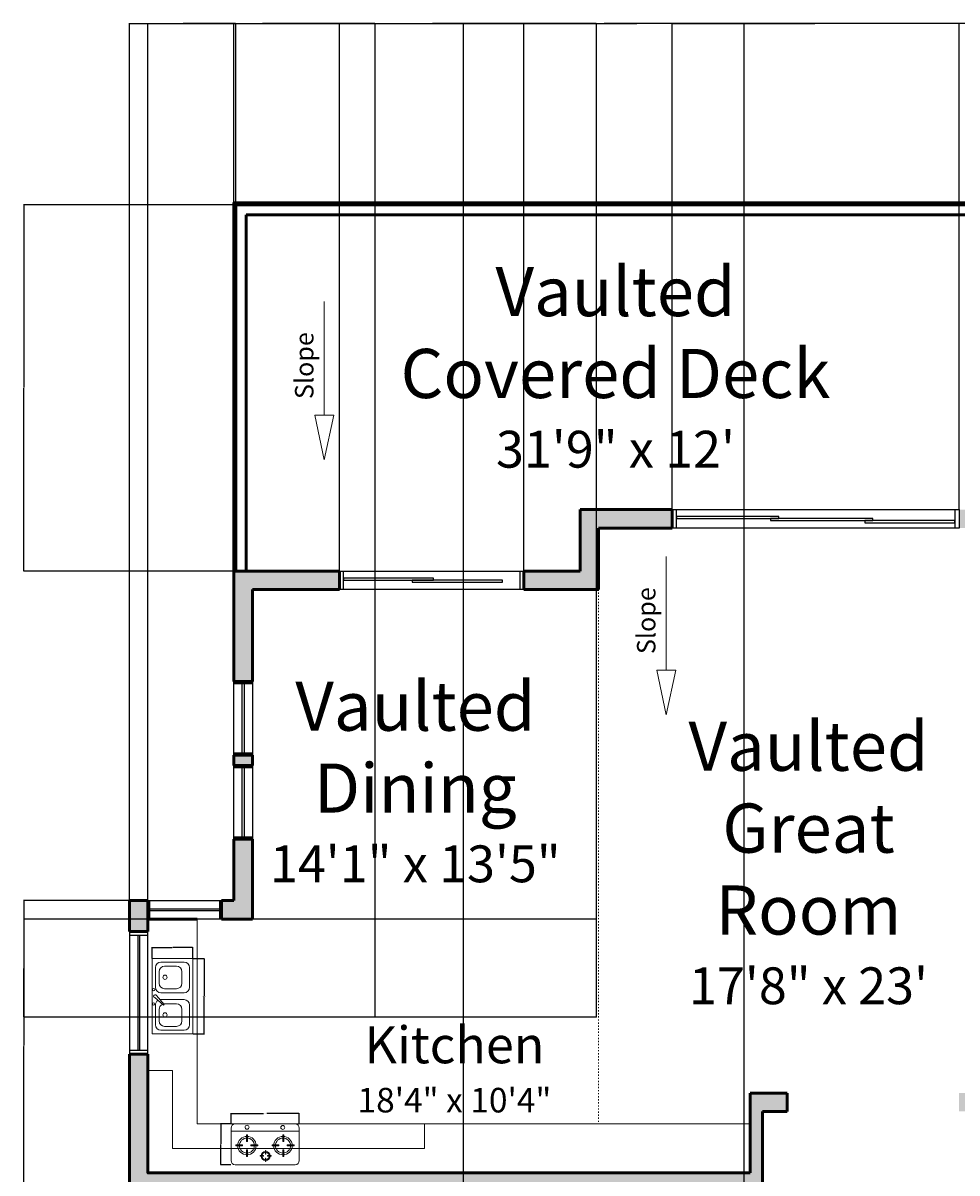
# Model space of a CAD drawing. Units: inches. Extents: x 296 to 2116, y 330 to 1460.
# Tile 3 of 9: x 296 to 752, y 898 to 1460. Entities that reach past the tile are written whole.
import ezdxf

# ---------------------------------------------------------------- set-up
doc = ezdxf.new("R2010")
doc.units = ezdxf.units.IN
doc.linetypes.add('ACAD_ISO03W100', pattern=[30, 12, -18])
for name, color, linetype, lineweight in [('A-ANNO-DIMS', 2, 'Continuous', 18), ('A-ANNO-SYMB', 2, 'Continuous', 18), ('A-ANNO-TEXT', 7, 'Continuous', 18), ('A-AREA-IDEN', 7, 'Continuous', 25), ('A-DOOR', 3, 'Continuous', 25), ('A-FLOR-FIXT', 8, 'Continuous', 18), ('A-FLOR-OVHD', 132, 'ACAD_ISO03W100', 18), ('A-GLAZ', 4, 'Continuous', 25), ('A-WALL', 7, 'Continuous', 50), ('A-WALL-PATT', 8, 'Continuous', 13)]:
    doc.layers.add(name, color=color, linetype=linetype, lineweight=lineweight)
doc.styles.get("Standard").update_dxf_attribs({"font": 'arial.ttf'})
doc.dimstyles.get("Standard").update_dxf_attribs({"dimtxt": 0.18, "dimasz": 0.18, "dimexe": 0.18, "dimexo": 0.0625, "dimgap": 0.09, "dimtad": 0, "dimtih": 1, "dimtoh": 1, "dimdec": 4, "dimzin": 0, "dimdsep": 46, "dimtxsty": 'Standard', "dimcen": 0.09, "dimadec": 0, "dimazin": 0, "dimtfac": 1, "dimtdec": 4, "dimtofl": 0, "dimtmove": 0, "dimatfit": 3, "dimfxl": 1, "dimtolj": 1, "dimtzin": 0, "dimarcsym": 0})

# ---------------------------------------------------------------- blocks, each defined once
blk = doc.blocks.new('A$C4ACA465A')
for p, q in [((0, 600), (0, 0)), ((0, 600), (1100, 600)), ((130, 550), (420, 550)), ((529, 561), (416, 432)), ((428, 421), (559, 534)), ((680, 550), (970, 550)), ((1100, 600), (1100, 0)), ((50, 470), (50, 130)), ((108, 416), (108, 241)), ((188, 496), (357, 496)), ((416, 432), (428, 421)), ((437, 416), (437, 241)), ((500, 470), (500, 130)), ((600, 470), (600, 130)), ((660, 416), (660, 241)), ((740, 496), (909, 496)), ((989, 416), (989, 241)), ((1050, 470), (1050, 130)), ((130, 50), (420, 50)), ((188, 161), (357, 161)), ((680, 50), (970, 50)), ((740, 161), (909, 161)), ((0, 0), (1100, 0))]:
    blk.add_line(p, q)
for centre, radius in [((437, 574), 17.2), ((647, 574), 17.2), ((275, 410), 31.1), ((827, 410), 31.1)]:
    blk.add_circle(centre, radius)
for centre, radius, start, end in [((130, 470), 80, 90, 180), ((420, 470), 80, 32.6633, 90), ((550, 554), 21.9, 294.4719, 162.1402), ((680, 470), 80, 90, 180), ((970, 470), 80, 0, 90), ((188, 416), 80, 90, 180), ((357, 416), 80, 23.6053, 90), ((357, 416), 80, 0, 8.7069), ((420, 470), 80, 0, 8.948), ((740, 416), 80, 90, 180), ((909, 416), 80, 0, 90), ((188, 241), 80, 180, 270), ((357, 241), 80, 270, 0), ((740, 241), 80, 180, 270), ((909, 241), 80, 270, 0), ((130, 130), 80, 180, 270), ((420, 130), 80, 270, 0), ((680, 130), 80, 180, 270), ((970, 130), 80, 270, 0)]:
    blk.add_arc(centre, radius, start, end)
blk = doc.blocks.new('A$C2A3C6842')
for p, q in [((0, 45), (0, 387)), ((45, 432), (675, 432)), ((352, 363), (352, 399)), ((352, 399), (357, 399)), ((357, 399), (357, 363)), ((720, 387), (720, 45)), ((162, 347), (173, 347)), ((162, 276), (162, 347)), ((173, 276), (162, 276)), ((173, 347), (173, 276)), ((298, 342), (298, 336)), ((334, 342), (298, 342)), ((298, 336), (334, 336)), ((334, 336), (334, 342)), ((357, 363), (352, 363)), ((357, 319), (352, 319)), ((352, 319), (352, 283)), ((352, 283), (357, 283)), ((357, 283), (357, 319)), ((379, 336), (379, 342)), ((379, 342), (414, 342)), ((414, 336), (379, 336)), ((414, 342), (414, 336)), ((545, 347), (556, 347)), ((545, 276), (545, 347)), ((556, 276), (545, 276)), ((556, 347), (556, 276)), ((55, 233), (55, 221)), ((127, 233), (55, 233)), ((55, 221), (127, 221)), ((127, 221), (127, 233)), ((173, 187), (162, 187)), ((162, 187), (162, 115)), ((173, 115), (173, 187)), ((216, 221), (216, 233)), ((216, 233), (287, 233)), ((287, 221), (216, 221)), ((287, 233), (287, 221)), ((438, 233), (438, 221)), ((510, 233), (438, 233)), ((438, 221), (510, 221)), ((510, 221), (510, 233)), ((556, 187), (545, 187)), ((545, 187), (545, 115)), ((556, 115), (556, 187)), ((598, 233), (670, 233)), ((598, 221), (598, 233)), ((670, 221), (598, 221)), ((670, 233), (670, 221)), ((1, 77), (720, 77)), ((162, 115), (173, 115)), ((545, 115), (556, 115)), ((675, 0), (45, 0))]:
    blk.add_line(p, q)
at = {"extrusion": (0, -1e-16, -1)}
for centre, major_axis, start_param, end_param in [((45, 387), (31.8, 31.8), 3.926991, 5.497787), ((172, 230), (-97.3, 0.1), -0.001099, 6.282086), ((552, 230), (-97.3, 0.1), -0.001099, 6.282086), ((174, 39), (-14.8, 14.8), 5.497787, 11.780972)]:
    blk.add_ellipse(centre, major_axis=major_axis, ratio=1, start_param=start_param, end_param=end_param, dxfattribs=at)
at = {"extrusion": (-1e-16, -1e-16, -1)}
blk.add_ellipse((355, 340), major_axis=(48.7, 0.1), ratio=1, start_param=3.144125, end_param=9.42731, dxfattribs=at)
at = {"extrusion": (-1e-16, 0, -1)}
for centre, major_axis, start_param, end_param in [((355, 340), (-39.7, 0), -0.000334, 6.282851), ((45, 45), (-31.8, 31.8), 3.926991, 5.497787)]:
    blk.add_ellipse(centre, major_axis=major_axis, ratio=1, start_param=start_param, end_param=end_param, dxfattribs=at)
at = {"extrusion": (0, 1e-16, -1)}
blk.add_ellipse((675, 387), major_axis=(-31.8, 31.8), ratio=1, start_param=0.785398, end_param=2.356194, dxfattribs=at)
at = {"extrusion": (-1e-16, -4e-16, -1)}
for centre in [(172, 230), (552, 230)]:
    blk.add_ellipse(centre, major_axis=(-79.3, 0), ratio=1, start_param=-0.0002116186602152, end_param=6.282973688519371, dxfattribs=at)
at = {"extrusion": (2e-16, -2e-16, -1)}
blk.add_ellipse((551, 36), major_axis=(14.8, 14.8), ratio=1, start_param=3.926991, end_param=10.210176, dxfattribs=at)
at = {"extrusion": (-2e-16, 1e-16, -1)}
blk.add_ellipse((675, 45), major_axis=(31.8, 31.8), ratio=1, start_param=0.785398, end_param=2.356194, dxfattribs=at)
at = {"text_generation_flag": 4, "flags": 9}
for tag in ['XSIZE', 'YSIZE']:
    blk.add_attdef(tag, (361, 265), '', height=0.45, rotation=180, dxfattribs=at)
blk = doc.blocks.new('SLOPE-ARROW')
blk.add_line((739.99, 662.71), (684.54, 662.71))
blk.add_lwpolyline([(662.67, 662.71), (684.54, 658.1), (684.54, 667.32)], close=True)
blk = doc.blocks.new('*D41')
at = {"layer": 'A-ANNO-DIMS', "color": 0, "lineweight": -2, "transparency": 16777216}
for p, q in [((378.58, 1002.67), (384.2, 1002.67)), ((384.02, 1002.49), (384.02, 984.52)), ((384.02, 966.18), (384.02, 984.15)), ((378.58, 966), (384.2, 966))]:
    blk.add_line(p, q, dxfattribs=at)
at = {"layer": 'A-ANNO-DIMS', "color": 0, "transparency": 16777216}
for points in [[(383.99, 1002.49), (384.05, 1002.49), (384.02, 1002.67)], [(383.99, 966.18), (384.05, 966.18), (384.02, 966)]]:
    blk.add_solid(points, dxfattribs=at)
at = {"layer": 'Defpoints', "color": 0, "transparency": 16777216}
for p in [(378.52, 1002.67), (384.02, 1002.67), (378.52, 966)]:
    blk.add_point(p, dxfattribs=at)
at = {"layer": 'A-ANNO-DIMS', "color": 0, "transparency": 16777216, "insert": (384.02, 984.33), "char_height": 0.18, "attachment_point": 5}
blk.add_mtext('\\A1;KITCHEN SINK 37', dxfattribs=at)
blk = doc.blocks.new('*D42')
at = {"layer": 'A-ANNO-DIMS', "color": 0, "lineweight": -2, "transparency": 16777216}
for p, q in [((358.52, 1002.73), (358.52, 1008.35)), ((358.7, 1008.17), (368.3, 1008.17)), ((378.34, 1008.17), (368.74, 1008.17)), ((378.52, 1002.73), (378.52, 1008.35))]:
    blk.add_line(p, q, dxfattribs=at)
at = {"layer": 'A-ANNO-DIMS', "color": 0, "transparency": 16777216}
for points in [[(358.7, 1008.2), (358.7, 1008.14), (358.52, 1008.17)], [(378.34, 1008.2), (378.34, 1008.14), (378.52, 1008.17)]]:
    blk.add_solid(points, dxfattribs=at)
at = {"layer": 'Defpoints', "color": 0, "transparency": 16777216}
for p in [(358.52, 1008.17), (358.52, 1002.67), (378.52, 1002.67)]:
    blk.add_point(p, dxfattribs=at)
at = {"layer": 'A-ANNO-DIMS', "color": 0, "transparency": 16777216, "insert": (368.52, 1008.17), "char_height": 0.18, "attachment_point": 5}
blk.add_mtext('\\A1;20', dxfattribs=at)
blk = doc.blocks.new('*D43')
at = {"layer": 'A-ANNO-DIMS', "color": 0, "lineweight": -2, "transparency": 16777216}
for p, q in [((397.09, 922.06), (397.09, 927.18)), ((397.27, 927), (412.88, 927)), ((430.25, 927), (414.64, 927)), ((430.43, 922.06), (430.43, 927.18))]:
    blk.add_line(p, q, dxfattribs=at)
at = {"layer": 'A-ANNO-DIMS', "color": 0, "transparency": 16777216}
for points in [[(397.27, 927.03), (397.27, 926.97), (397.09, 927)], [(430.25, 927.03), (430.25, 926.97), (430.43, 927)]]:
    blk.add_solid(points, dxfattribs=at)
at = {"layer": 'Defpoints', "color": 0, "transparency": 16777216}
for p in [(397.09, 927), (397.09, 922), (430.43, 922)]:
    blk.add_point(p, dxfattribs=at)
at = {"layer": 'A-ANNO-DIMS', "color": 0, "transparency": 16777216, "insert": (413.76, 927), "char_height": 0.18, "attachment_point": 5}
blk.add_mtext('\\A1;COOKTOP 33', dxfattribs=at)
blk = doc.blocks.new('*D44')
at = {"layer": 'A-ANNO-DIMS', "color": 0, "lineweight": -2, "transparency": 16777216}
for p, q in [((397.03, 922), (391.91, 922)), ((392.09, 921.82), (392.09, 912.18)), ((392.09, 902.18), (392.09, 911.82)), ((397.03, 902), (391.91, 902))]:
    blk.add_line(p, q, dxfattribs=at)
at = {"layer": 'A-ANNO-DIMS', "color": 0, "transparency": 16777216}
for points in [[(392.06, 921.82), (392.12, 921.82), (392.09, 922)], [(392.06, 902.18), (392.12, 902.18), (392.09, 902)]]:
    blk.add_solid(points, dxfattribs=at)
at = {"layer": 'Defpoints', "color": 0, "transparency": 16777216}
for p in [(397.09, 922), (392.09, 902), (397.09, 902)]:
    blk.add_point(p, dxfattribs=at)
at = {"layer": 'A-ANNO-DIMS', "color": 0, "transparency": 16777216, "insert": (392.09, 912), "char_height": 0.18, "attachment_point": 5}
blk.add_mtext('\\A1;20', dxfattribs=at)
blk = doc.blocks.new('*D45')
at = {"layer": 'A-ANNO-DIMS', "color": 0, "lineweight": -2, "transparency": 16777216}
for p, q in [((1156.58, 1407.95), (1235.3, 1407.95)), ((1235.12, 1407.77), (1235.12, 895.66)), ((1235.12, 383.18), (1235.12, 895.29)), ((609.63, 383), (1235.3, 383))]:
    blk.add_line(p, q, dxfattribs=at)
at = {"layer": 'A-ANNO-DIMS', "color": 0, "transparency": 16777216}
for points in [[(1235.09, 1407.77), (1235.15, 1407.77), (1235.12, 1407.95)], [(1235.09, 383.18), (1235.15, 383.18), (1235.12, 383)]]:
    blk.add_solid(points, dxfattribs=at)
at = {"layer": 'Defpoints', "color": 0, "transparency": 16777216}
for p in [(1156.52, 1407.95), (1235.12, 1407.95), (609.57, 383)]:
    blk.add_point(p, dxfattribs=at)
at = {"layer": 'A-ANNO-DIMS', "color": 0, "transparency": 16777216, "insert": (1235.12, 895.48), "char_height": 0.18, "attachment_point": 5}
blk.add_mtext('\\A1;1025', dxfattribs=at)
blk = doc.blocks.new('*D46')
at = {"layer": 'A-ANNO-DIMS', "color": 0, "lineweight": -2, "transparency": 16777216}
for p, q in [((399.52, 1371.02), (399.52, 1459.73)), ((399.7, 1459.55), (595.23, 1459.55)), ((791.34, 1459.55), (595.81, 1459.55)), ((791.52, 1372.02), (791.52, 1459.73))]:
    blk.add_line(p, q, dxfattribs=at)
at = {"layer": 'A-ANNO-DIMS', "color": 0, "transparency": 16777216}
for points in [[(399.7, 1459.58), (399.7, 1459.52), (399.52, 1459.55)], [(791.34, 1459.58), (791.34, 1459.52), (791.52, 1459.55)]]:
    blk.add_solid(points, dxfattribs=at)
at = {"layer": 'Defpoints', "color": 0, "transparency": 16777216}
for p in [(791.52, 1459.55), (399.52, 1370.95), (791.52, 1371.95)]:
    blk.add_point(p, dxfattribs=at)
at = {"layer": 'A-ANNO-DIMS', "color": 0, "transparency": 16777216, "insert": (595.52, 1459.55), "char_height": 0.18, "attachment_point": 5}
blk.add_mtext('\\A1;392', dxfattribs=at)
blk = doc.blocks.new('*D49')
at = {"layer": 'A-ANNO-DIMS', "color": 0, "lineweight": -2, "transparency": 16777216}
for p, q in [((347.52, 1031.06), (347.52, 1459.73)), ((347.7, 1459.55), (373.3, 1459.55)), ((399.34, 1459.55), (373.74, 1459.55)), ((399.52, 1371.02), (399.52, 1459.73))]:
    blk.add_line(p, q, dxfattribs=at)
at = {"layer": 'A-ANNO-DIMS', "color": 0, "transparency": 16777216}
for points in [[(347.7, 1459.58), (347.7, 1459.52), (347.52, 1459.55)], [(399.34, 1459.58), (399.34, 1459.52), (399.52, 1459.55)]]:
    blk.add_solid(points, dxfattribs=at)
at = {"layer": 'Defpoints', "color": 0, "transparency": 16777216}
for p in [(399.52, 1459.55), (399.52, 1370.95), (347.52, 1031)]:
    blk.add_point(p, dxfattribs=at)
at = {"layer": 'A-ANNO-DIMS', "color": 0, "transparency": 16777216, "insert": (373.52, 1459.55), "char_height": 0.18, "attachment_point": 5}
blk.add_mtext('\\A1;52', dxfattribs=at)
blk = doc.blocks.new('*D58')
at = {"layer": 'A-ANNO-DIMS', "color": 0, "lineweight": -2, "transparency": 16777216}
for p, q in [((347.46, 1031), (295.74, 1031)), ((295.92, 1030.82), (295.92, 960.18)), ((295.92, 889.18), (295.92, 959.82)), ((347.46, 889), (295.74, 889))]:
    blk.add_line(p, q, dxfattribs=at)
at = {"layer": 'A-ANNO-DIMS', "color": 0, "transparency": 16777216}
for points in [[(295.89, 1030.82), (295.95, 1030.82), (295.92, 1031)], [(295.89, 889.18), (295.95, 889.18), (295.92, 889)]]:
    blk.add_solid(points, dxfattribs=at)
at = {"layer": 'Defpoints', "color": 0, "transparency": 16777216}
for p in [(295.92, 1031), (347.52, 1031), (347.52, 889)]:
    blk.add_point(p, dxfattribs=at)
at = {"layer": 'A-ANNO-DIMS', "color": 0, "transparency": 16777216, "insert": (295.92, 960), "char_height": 0.18, "attachment_point": 5}
blk.add_mtext('\\A1;142', dxfattribs=at)
blk = doc.blocks.new('*D59')
at = {"layer": 'A-ANNO-DIMS', "color": 0, "lineweight": -2, "transparency": 16777216}
for p, q in [((399.46, 1370.95), (295.74, 1370.95)), ((295.92, 1370.77), (295.92, 1281.66)), ((295.92, 1192.18), (295.92, 1281.29)), ((399.46, 1192), (295.74, 1192))]:
    blk.add_line(p, q, dxfattribs=at)
at = {"layer": 'A-ANNO-DIMS', "color": 0, "transparency": 16777216}
for points in [[(295.89, 1370.77), (295.95, 1370.77), (295.92, 1370.95)], [(295.89, 1192.18), (295.95, 1192.18), (295.92, 1192)]]:
    blk.add_solid(points, dxfattribs=at)
at = {"layer": 'Defpoints', "color": 0, "transparency": 16777216}
for p in [(399.52, 1370.95), (295.92, 1192), (399.52, 1192)]:
    blk.add_point(p, dxfattribs=at)
at = {"layer": 'A-ANNO-DIMS', "color": 0, "transparency": 16777216, "insert": (295.92, 1281.48), "char_height": 0.18, "attachment_point": 5}
blk.add_mtext('\\A1;178.96', dxfattribs=at)
blk = doc.blocks.new('*D66')
at = {"layer": 'A-ANNO-DIMS', "color": 0, "lineweight": -2, "transparency": 16777216}
for p, q in [((510.57, 889.06), (510.57, 1459.73)), ((510.75, 1459.55), (578.79, 1459.55)), ((647.39, 1459.55), (579.35, 1459.55)), ((647.57, 889.06), (647.57, 1459.73))]:
    blk.add_line(p, q, dxfattribs=at)
at = {"layer": 'A-ANNO-DIMS', "color": 0, "transparency": 16777216}
for points in [[(510.75, 1459.58), (510.75, 1459.52), (510.57, 1459.55)], [(647.39, 1459.58), (647.39, 1459.52), (647.57, 1459.55)]]:
    blk.add_solid(points, dxfattribs=at)
at = {"layer": 'Defpoints', "color": 0, "transparency": 16777216}
for p in [(647.57, 1459.55), (510.57, 889), (647.57, 889)]:
    blk.add_point(p, dxfattribs=at)
at = {"layer": 'A-ANNO-DIMS', "color": 0, "transparency": 16777216, "insert": (579.07, 1459.55), "char_height": 0.18, "attachment_point": 5}
blk.add_mtext('\\A1;137', dxfattribs=at)
blk = doc.blocks.new('*D78')
at = {"layer": 'A-ANNO-DIMS', "color": 0, "lineweight": -2, "transparency": 16777216}
for p, q in [((398.52, 1192.06), (398.52, 1459.73)), ((398.7, 1459.55), (593.06, 1459.55)), ((788.34, 1459.55), (593.99, 1459.55)), ((788.52, 1213.06), (788.52, 1459.73))]:
    blk.add_line(p, q, dxfattribs=at)
at = {"layer": 'A-ANNO-DIMS', "color": 0, "transparency": 16777216}
for points in [[(398.7, 1459.58), (398.7, 1459.52), (398.52, 1459.55)], [(788.34, 1459.58), (788.34, 1459.52), (788.52, 1459.55)]]:
    blk.add_solid(points, dxfattribs=at)
at = {"layer": 'Defpoints', "color": 0, "transparency": 16777216}
for p in [(788.52, 1459.55), (788.52, 1213), (398.52, 1192)]:
    blk.add_point(p, dxfattribs=at)
at = {"layer": 'A-ANNO-DIMS', "color": 0, "transparency": 16777216, "insert": (593.52, 1459.55), "char_height": 0.18, "attachment_point": 5}
blk.add_mtext('\\A1;390.00', dxfattribs=at)
blk = doc.blocks.new('*D86')
at = {"layer": 'A-ANNO-DIMS', "color": 0, "lineweight": -2, "transparency": 16777216}
for p, q in [((356.52, 1022.06), (356.52, 1459.73)), ((356.7, 1459.55), (411.57, 1459.55)), ((467.34, 1459.55), (412.48, 1459.55)), ((467.52, 1022.06), (467.52, 1459.73))]:
    blk.add_line(p, q, dxfattribs=at)
at = {"layer": 'A-ANNO-DIMS', "color": 0, "transparency": 16777216}
for points in [[(356.7, 1459.58), (356.7, 1459.52), (356.52, 1459.55)], [(467.34, 1459.58), (467.34, 1459.52), (467.52, 1459.55)]]:
    blk.add_solid(points, dxfattribs=at)
at = {"layer": 'Defpoints', "color": 0, "transparency": 16777216}
for p in [(467.52, 1459.55), (356.52, 1022), (467.52, 1022)]:
    blk.add_point(p, dxfattribs=at)
at = {"layer": 'A-ANNO-DIMS', "color": 0, "transparency": 16777216, "insert": (412.02, 1459.55), "char_height": 0.18, "attachment_point": 5}
blk.add_mtext('\\A1;111.00', dxfattribs=at)
blk = doc.blocks.new('*D87')
at = {"layer": 'A-ANNO-DIMS', "color": 0, "lineweight": -2, "transparency": 16777216}
for p, q in [((467.52, 974.06), (467.52, 1459.73)), ((467.7, 1459.55), (521.07, 1459.55)), ((575.34, 1459.55), (521.98, 1459.55)), ((575.52, 974.06), (575.52, 1459.73))]:
    blk.add_line(p, q, dxfattribs=at)
at = {"layer": 'A-ANNO-DIMS', "color": 0, "transparency": 16777216}
for points in [[(467.7, 1459.58), (467.7, 1459.52), (467.52, 1459.55)], [(575.34, 1459.58), (575.34, 1459.52), (575.52, 1459.55)]]:
    blk.add_solid(points, dxfattribs=at)
at = {"layer": 'Defpoints', "color": 0, "transparency": 16777216}
for p in [(575.52, 1459.55), (467.52, 974), (575.52, 974)]:
    blk.add_point(p, dxfattribs=at)
at = {"layer": 'A-ANNO-DIMS', "color": 0, "transparency": 16777216, "insert": (521.52, 1459.55), "char_height": 0.18, "attachment_point": 5}
blk.add_mtext('\\A1;108.00', dxfattribs=at)
blk = doc.blocks.new('*D88')
at = {"layer": 'A-ANNO-DIMS', "color": 0, "lineweight": -2, "transparency": 16777216}
for p, q in [((575.46, 1022), (295.74, 1022)), ((295.92, 1021.82), (295.92, 998.18)), ((295.92, 974.18), (295.92, 997.82)), ((575.46, 974), (295.74, 974))]:
    blk.add_line(p, q, dxfattribs=at)
at = {"layer": 'A-ANNO-DIMS', "color": 0, "transparency": 16777216}
for points in [[(295.89, 1021.82), (295.95, 1021.82), (295.92, 1022)], [(295.89, 974.18), (295.95, 974.18), (295.92, 974)]]:
    blk.add_solid(points, dxfattribs=at)
at = {"layer": 'Defpoints', "color": 0, "transparency": 16777216}
for p in [(295.92, 1022), (575.52, 1022), (575.52, 974)]:
    blk.add_point(p, dxfattribs=at)
at = {"layer": 'A-ANNO-DIMS', "color": 0, "transparency": 16777216, "insert": (295.92, 998), "char_height": 0.18, "attachment_point": 5}
blk.add_mtext('\\A1;48.00', dxfattribs=at)
blk = doc.blocks.new('*D103')
at = {"layer": 'A-ANNO-DIMS', "color": 0, "lineweight": -2, "transparency": 16777216}
for p, q in [((450.022265, 1192.061588), (450.022265, 1459.734098)), ((450.202265, 1459.554098), (494.628868, 1459.554098)), ((539.842265, 1459.554098), (495.415662, 1459.554098)), ((540.022265, 1192.061588), (540.022265, 1459.734098))]:
    blk.add_line(p, q, dxfattribs=at)
at = {"layer": 'A-ANNO-DIMS', "color": 0, "transparency": 16777216}
for points in [[(450.202265, 1459.584098), (450.202265, 1459.524098), (450.022265, 1459.554098)], [(539.842265, 1459.584098), (539.842265, 1459.524098), (540.022265, 1459.554098)]]:
    blk.add_solid(points, dxfattribs=at)
at = {"layer": 'Defpoints', "color": 0, "transparency": 16777216}
for p in [(540.022265, 1459.554098), (450.022265, 1191.999088), (540.022265, 1191.999088)]:
    blk.add_point(p, dxfattribs=at)
at = {"layer": 'A-ANNO-DIMS', "color": 0, "transparency": 16777216, "insert": (495.022265, 1459.554098), "char_height": 0.18, "attachment_point": 5}
blk.add_mtext('\\A1;90.00', dxfattribs=at)
blk = doc.blocks.new('*D104')
at = {"layer": 'A-ANNO-DIMS', "color": 0, "lineweight": -2, "transparency": 16777216}
for p, q in [((612.52, 1222.06), (612.52, 1459.73)), ((612.7, 1459.55), (682.07, 1459.55)), ((752.34, 1459.55), (682.98, 1459.55)), ((752.52, 1222.06), (752.52, 1459.73))]:
    blk.add_line(p, q, dxfattribs=at)
at = {"layer": 'A-ANNO-DIMS', "color": 0, "transparency": 16777216}
for points in [[(612.7, 1459.58), (612.7, 1459.52), (612.52, 1459.55)], [(752.34, 1459.58), (752.34, 1459.52), (752.52, 1459.55)]]:
    blk.add_solid(points, dxfattribs=at)
at = {"layer": 'Defpoints', "color": 0, "transparency": 16777216}
for p in [(752.52, 1459.55), (612.52, 1222), (752.52, 1222)]:
    blk.add_point(p, dxfattribs=at)
at = {"layer": 'A-ANNO-DIMS', "color": 0, "transparency": 16777216, "insert": (682.52, 1459.55), "char_height": 0.18, "attachment_point": 5}
blk.add_mtext('\\A1;140.00', dxfattribs=at)

msp = doc.modelspace()

# ---------------------------------------------------------------- hatches: boundary and pattern name
at = {"layer": 'A-WALL-PATT'}
h = msp.add_hatch(color=256, dxfattribs=at)
h.dxf.hatch_style = 1
h.paths.add_polyline_path([(656.5723, 927.9991), (668.5723, 927.9991), (668.5723, 936.9991), (650.5723, 936.9991), (650.5723, 897.9991), (356.5223, 897.9991), (356.5223, 955.9991), (347.5223, 955.9991), (347.5223, 888.9991), (423.5723, 888.9991), (423.5723, 766.9991), (432.5723, 766.9991), (432.5723, 834.9991), (453.5723, 834.9991), (468.5723, 834.9991), (468.5723, 840.9991), (432.5723, 840.9991), (432.5723, 888.9991), (504.5723, 888.9991), (504.5723, 840.9991), (504.5723, 834.9991), (531.6223, 834.9991), (531.6223, 768.5344), (527.8443, 764.7564), (530.6728, 761.928), (532.087, 760.5138), (540.5723, 768.9991), (598.0723, 768.9991), (598.0723, 777.9991), (601.8223, 777.9991), (601.8223, 782.1991), (601.8223, 783.9991), (598.0723, 783.9991), (598.0723, 798.9991), (592.0723, 798.9991), (592.0723, 774.9991), (537.6223, 774.9991), (537.6223, 834.9991), (592.0723, 834.9991), (592.0723, 828.9991), (598.0723, 828.9991), (598.0723, 834.9991), (647.5723, 834.9991), (647.5723, 828.9991), (656.5723, 828.9991), (656.5723, 846.9991), (650.5723, 846.9991), (647.5723, 846.9991), (647.5723, 840.9991), (510.5723, 840.9991), (510.5723, 888.9991), (647.5723, 888.9991), (647.5723, 882.9991), (656.5723, 882.9991)])
h.paths.add_polyline_path([(432.5723, 730.9991), (496.5723, 730.9991), (496.5723, 724.9991), (502.5723, 724.9991), (502.5723, 730.9991), (506.6311, 735.058), (502.3885, 739.3006), (500.087, 736.9991), (432.5723, 736.9991), (432.5723, 742.9991), (423.5723, 742.9991), (423.5723, 641.9991), (490.5723, 641.9991), (490.5723, 597.9991), (531.5723, 597.9991), (531.5723, 606.9991), (499.5723, 606.9991), (499.5723, 650.9991), (502.5723, 650.9991), (502.5723, 659.9991), (496.5723, 659.9991), (493.5723, 659.9991), (493.5723, 650.9991), (432.5723, 650.9991)])
h.paths.add_polyline_path([(656.5723, 689.4991), (662.5473, 689.4991), (662.5473, 698.4991), (656.5723, 698.4991), (656.5723, 789.9991), (647.5723, 789.9991), (647.5723, 783.9991), (643.8223, 783.9991), (643.8223, 777.9991), (647.5723, 777.9991), (647.5723, 606.9991), (615.5723, 606.9991), (615.5723, 597.9991), (656.5723, 597.9991)])
h.paths.add_polyline_path([(761.5223, 780.9541), (797.5223, 780.9541), (797.5223, 789.9541), (761.5223, 789.9541), (761.5223, 858.9541), (797.5223, 858.9541), (797.5223, 867.9541), (752.5223, 867.9541), (752.5223, 698.4991), (746.5473, 698.4991), (746.5473, 694.2991), (746.5473, 689.4991), (752.5223, 689.4991), (752.5223, 624.9541), (761.5223, 624.9541)])
h.paths.add_polyline_path([(1102.5223, 795.9541), (1093.5223, 795.9541), (1093.5223, 789.9541), (1063.5223, 789.9541), (881.5223, 789.9541), (881.5223, 837.9541), (911.5223, 837.9541), (911.5223, 849.9541), (907.5223, 849.9541), (905.5223, 849.9541), (905.5223, 843.9541), (845.5223, 843.9541), (845.5223, 834.9541), (849.0223, 834.9541), (851.5223, 834.9541), (851.5223, 837.9541), (875.5223, 837.9541), (875.5223, 789.9541), (851.5223, 789.9541), (851.5223, 792.9541), (845.5223, 792.9541), (845.5223, 789.9541), (833.5223, 789.9541), (833.5223, 785.1541), (833.5223, 780.9541), (1049.5223, 780.9541), (1049.5223, 726.9541), (1053.7223, 726.9541), (1058.5223, 726.9541), (1058.5223, 780.9541), (1102.5223, 780.9541)])
h.paths.add_polyline_path([(761.5223, 588.9541), (752.5223, 588.9541), (752.5223, 564.9541), (761.5223, 564.9541)])
h.paths.add_polyline_path([(809.5223, 480.9541), (761.5223, 480.9541), (761.5223, 528.9541), (752.5223, 528.9541), (752.5223, 471.9541), (809.5223, 471.9541)])
h.paths.add_polyline_path([(1058.5223, 684.9541), (1049.5223, 684.9541), (1049.5223, 480.9541), (1001.5223, 480.9541), (1001.5223, 476.4541), (1001.5223, 471.9541), (1058.5223, 471.9541)])
h.paths.add_polyline_path([(794.5223, 1013.9991), (800.5223, 1013.9991), (800.5223, 1019.9991), (794.5223, 1019.9991), (794.5223, 1296.9541), (785.5223, 1296.9541), (785.5223, 1221.9991), (752.5223, 1221.9991), (752.5223, 1212.9991), (788.5223, 1212.9991), (788.5223, 936.9991), (752.5223, 936.9991), (752.5223, 927.9991), (794.5223, 927.9991)])
h.paths.add_polyline_path([(450.0223, 1191.9991), (398.5223, 1191.9991), (398.5223, 1137.9991), (407.5223, 1137.9991), (407.5223, 1182.9991), (450.0223, 1182.9991)])
h.paths.add_polyline_path([(576.5223, 1212.9991), (612.5223, 1212.9991), (612.5223, 1221.9991), (567.5223, 1221.9991), (567.5223, 1191.9991), (540.0223, 1191.9991), (540.0223, 1182.9991), (576.5223, 1182.9991)])
h.paths.add_polyline_path([(407.5223, 1060.9991), (398.5223, 1060.9991), (398.5223, 1030.9991), (392.5223, 1030.9991), (392.5223, 1021.9991), (407.5223, 1021.9991)])
h.paths.add_polyline_path([(356.5223, 1030.9991), (347.5223, 1030.9991), (347.5223, 1015.9991), (356.5223, 1015.9991), (356.5223, 1021.9991)])
h.paths.add_polyline_path([(788.5223, 1129.9991), (770.0334, 1131.3572, 0.43585667), (767.8869, 1129.3626), (767.8869, 1108.3618, 0.31855172), (769.8942, 1105.5308), (788.5223, 1098.9991)], flags=17)
h.paths.add_polyline_path([(788.5223, 1050.9991), (769.8942, 1044.4674, 0.31855172), (767.8869, 1041.6364), (767.8869, 1020.6356, 0.43585667), (770.0334, 1018.641), (788.5223, 1019.9991)], flags=17)
h.paths.add_polyline_path([(893.5223, 1066.9541), (851.5223, 1066.9541), (851.5223, 1069.9541), (845.5223, 1069.9541), (845.5223, 1019.9991), (839.5223, 1019.9991), (839.5223, 1013.9991), (845.5223, 1013.9991), (845.5223, 891.9541), (863.5223, 891.9541), (863.5223, 897.9541), (851.5223, 897.9541), (851.5223, 927.9541), (905.5223, 927.9541), (905.5223, 897.9541), (893.5223, 897.9541), (893.5223, 891.9541), (905.5223, 891.9541), (905.5223, 885.9541), (911.5223, 885.9541), (911.5223, 927.9541), (1030.5223, 927.9541), (1030.5223, 936.9541), (1013.5223, 936.9541), (1013.5223, 996.9541), (1093.5223, 996.9541), (1093.5223, 936.9541), (1066.5223, 936.9541), (1066.5223, 927.9541), (1093.5223, 927.9541), (1093.5223, 921.9541), (1102.5223, 921.9541), (1102.5223, 1013.9541), (1093.5223, 1013.9541), (1093.5223, 1002.9541), (1013.5223, 1002.9541), (1013.5223, 1060.9541), (1013.5223, 1066.9541), (1007.5223, 1066.9541), (1007.5223, 1042.9541), (977.5223, 1042.9541), (977.5223, 1066.9541), (965.5223, 1066.9541), (965.5223, 1060.9541), (971.5223, 1060.9541), (971.5223, 1036.9541), (1007.5223, 1036.9541), (1007.5223, 936.9541), (851.5223, 936.9541), (851.5223, 1060.9541), (893.5223, 1060.9541)])
h.paths.add_polyline_path([(851.5223, 1150.9541), (919.5223, 1150.9541), (919.5223, 1114.9541), (911.5223, 1114.9541), (911.5223, 1108.9541), (925.5223, 1108.9541), (925.5223, 1150.9541), (1007.5223, 1150.9541), (1007.5223, 1114.9541), (1013.5223, 1114.9541), (1013.5223, 1150.9541), (1046.5223, 1150.9541), (1046.5223, 1159.9541), (1007.5223, 1159.9541), (1007.5223, 1186.9541), (998.5223, 1186.9541), (998.5223, 1156.9541), (845.5223, 1156.9541), (845.5223, 1105.9541), (851.5223, 1105.9541)])
h.paths.add_polyline_path([(1102.5223, 1156.9541), (1102.5223, 1159.9541), (1088.5223, 1159.9541), (1088.5223, 1150.9541), (1093.5223, 1150.9541), (1093.5223, 1147.9541), (1102.5223, 1147.9541)])
h.paths.add_polyline_path([(1102.5223, 1111.9541), (1093.5223, 1111.9541), (1093.5223, 1066.9541), (1047.5223, 1066.9541), (1047.5223, 1030.9541), (1053.5223, 1030.9541), (1053.5223, 1060.9541), (1093.5223, 1060.9541), (1093.5223, 1049.9541), (1102.5223, 1049.9541)])
h.paths.add_polyline_path([(1102.5223, 837.9541), (1093.5223, 837.9541), (1093.5223, 831.9541), (1102.5223, 831.9541)], flags=17)
h.paths.add_polyline_path([(1102.5223, 879.9541), (1093.5223, 879.9541), (1093.5223, 873.9541), (1102.5223, 873.9541)])
h.paths.add_polyline_path([(839.5223, 1353.9541), (785.5223, 1353.9541), (785.5223, 1338.9541), (794.5223, 1338.9541), (794.5223, 1344.9541), (839.5223, 1344.9541)])
h.paths.add_polyline_path([(1007.5223, 1353.9541), (953.5223, 1353.9541), (953.5223, 1344.9541), (998.5223, 1344.9541), (998.5223, 1314.9541), (1007.5223, 1314.9541)])
h.paths.add_polyline_path([(917.5223, 1353.9541), (914.5223, 1353.9541), (914.5223, 1344.9541), (917.5223, 1344.9541)])
h.paths.add_polyline_path([(878.5223, 1353.9541), (875.5223, 1353.9541), (875.5223, 1344.9541), (878.5223, 1344.9541)])
h.paths.add_polyline_path([(1007.5223, 1278.9541), (998.5223, 1278.9541), (998.5223, 1222.9541), (1007.5223, 1222.9541)])
h.paths.add_polyline_path([(407.5223, 1101.9991), (398.5223, 1101.9991), (398.5223, 1096.9991), (407.5223, 1096.9991)])
h.paths.add_polyline_path([(560.5723, 606.9991), (557.5723, 606.9991), (557.5723, 597.9991), (560.5723, 597.9991)])
h.paths.add_polyline_path([(589.5723, 606.9991), (586.5723, 606.9991), (586.5723, 597.9991), (589.5723, 597.9991)])

# ---------------------------------------------------------------- linework, layer by layer
at = {"layer": 'A-DOOR'}
for p, q in [((614.5223, 1212.9991), (614.5223, 1221.9991)), ((750.5223, 1221.9991), (750.5223, 1212.9991)), ((452.0223, 1182.9991), (452.0223, 1191.9991)), ((538.0223, 1191.9991), (538.0223, 1182.9991))]:
    msp.add_line(p, q, dxfattribs=at)
for points in [[(752.5223, 1221.9991), (752.5223, 1212.9991), (612.5223, 1212.9991), (612.5223, 1221.9991)], [(614.5223, 1217.6372), (664.5223, 1217.6372), (664.5223, 1218.6372), (614.5223, 1218.6372)], [(660.4811, 1216.6372), (710.4811, 1216.6372), (710.4811, 1217.6372), (660.4811, 1217.6372)], [(706.5223, 1215.6372), (750.5223, 1215.6372), (750.5223, 1216.6372), (706.5223, 1216.6372)], [(540.0223, 1191.9991), (540.0223, 1182.9991), (450.0223, 1182.9991), (450.0223, 1191.9991)], [(452.0223, 1187.4991), (496.0223, 1187.4991), (496.0223, 1188.4991), (452.0223, 1188.4991)], [(485.5744, 1186.4991), (529.5744, 1186.4991), (529.5744, 1187.4991), (485.5744, 1187.4991)]]:
    msp.add_lwpolyline(points, close=True, dxfattribs=at)
at = {"layer": 'A-FLOR-FIXT'}
for p, q in [((368.5223, 947.9991), (356.5223, 947.9991)), ((491.5473, 909.9991), (491.5473, 921.9991))]:
    msp.add_line(p, q, dxfattribs=at)
for points in [[(380.5223, 1021.9991), (380.5223, 921.9991), (650.5723, 921.9991)], [(368.5223, 947.9991), (368.5223, 909.9991), (491.5473, 909.9991)]]:
    msp.add_lwpolyline(points, dxfattribs=at)
msp.add_lwpolyline([(467.5223, 973.9991), (575.5223, 973.9991), (575.5223, 1021.9991), (467.5223, 1021.9991)], close=True, dxfattribs=at)
at = {"layer": 'A-FLOR-OVHD', "ltscale": 0.05}
msp.add_line((576.5223, 1182.9991), (576.5223, 921.9991), dxfattribs=at)
at = {"layer": 'A-GLAZ'}
for p, q in [((398.5223, 1136.9991), (407.5223, 1136.9991)), ((402.5223, 1102.9991), (402.5223, 1136.9991)), ((403.5223, 1136.9991), (403.5223, 1102.9991)), ((407.5223, 1102.9991), (398.5223, 1102.9991)), ((398.5223, 1095.9991), (407.5223, 1095.9991)), ((402.5223, 1061.9991), (402.5223, 1095.9991)), ((403.5223, 1095.9991), (403.5223, 1061.9991)), ((407.5223, 1061.9991), (398.5223, 1061.9991)), ((357.5223, 1021.9991), (357.5223, 1030.9991)), ((391.5223, 1030.9991), (391.5223, 1021.9991)), ((357.5223, 1026.9991), (391.5223, 1026.9991)), ((391.5223, 1025.9991), (357.5223, 1025.9991)), ((356.5223, 1013.9991), (347.5223, 1013.9991)), ((351.5223, 1013.9991), (351.5223, 957.9991)), ((352.5223, 957.9991), (352.5223, 1013.9991)), ((347.5223, 957.9991), (356.5223, 957.9991))]:
    msp.add_line(p, q, dxfattribs=at)
for points in [[(407.5223, 1101.9991), (398.5223, 1101.9991), (398.5223, 1137.9991), (407.5223, 1137.9991)], [(407.5223, 1060.9991), (398.5223, 1060.9991), (398.5223, 1096.9991), (407.5223, 1096.9991)], [(356.5223, 1021.9991), (356.5223, 1030.9991), (392.5223, 1030.9991), (392.5223, 1021.9991)], [(356.5223, 955.9991), (356.5223, 1015.9991), (347.5223, 1015.9991), (347.5223, 955.9991)]]:
    msp.add_lwpolyline(points, close=True, dxfattribs=at)
at = {"layer": 'A-WALL'}
for p, q in [((785.5223, 1365.9541), (404.5223, 1365.9541)), ((404.5223, 1191.9991), (404.5223, 1365.9541)), ((567.5223, 1221.9991), (567.5223, 1191.9991)), ((612.5223, 1221.9991), (567.5223, 1221.9991)), ((612.5223, 1212.9991), (612.5223, 1221.9991)), ((576.5223, 1212.9991), (576.5223, 1182.9991)), ((612.5223, 1212.9991), (576.5223, 1212.9991)), ((450.0223, 1191.9991), (398.5223, 1191.9991)), ((398.5223, 1137.9991), (398.5223, 1191.9991)), ((450.0223, 1182.9991), (450.0223, 1191.9991)), ((567.5223, 1191.9991), (540.0223, 1191.9991)), ((540.0223, 1182.9991), (540.0223, 1191.9991)), ((450.0223, 1182.9991), (407.5223, 1182.9991)), ((407.5223, 1137.9991), (407.5223, 1182.9991)), ((576.5223, 1182.9991), (540.0223, 1182.9991)), ((398.5223, 1137.9991), (407.5223, 1137.9991)), ((407.5223, 1101.9991), (398.5223, 1101.9991)), ((398.5223, 1096.9991), (398.5223, 1101.9991)), ((407.5223, 1096.9991), (407.5223, 1101.9991)), ((407.5223, 1096.9991), (398.5223, 1096.9991)), ((398.5223, 1030.9991), (398.5223, 1060.9991)), ((398.5223, 1060.9991), (407.5223, 1060.9991)), ((407.5223, 1021.9991), (407.5223, 1060.9991)), ((347.5223, 1030.9991), (347.5223, 1015.9991)), ((356.5223, 1030.9991), (347.5223, 1030.9991)), ((356.5223, 1021.9991), (356.5223, 1030.9991)), ((398.5223, 1030.9991), (392.5223, 1030.9991)), ((392.5223, 1021.9991), (392.5223, 1030.9991)), ((380.5223, 1021.9991), (356.5223, 1021.9991)), ((407.5223, 1021.9991), (392.5223, 1021.9991)), ((356.5223, 1015.9991), (347.5223, 1015.9991)), ((356.5223, 955.9991), (347.5223, 955.9991)), ((347.5223, 955.9991), (347.5223, 888.9991)), ((650.5723, 897.9991), (650.5723, 936.9991)), ((668.5723, 936.9991), (650.5723, 936.9991)), ((668.5723, 936.9991), (668.5723, 927.9991)), ((668.5723, 927.9991), (656.5723, 927.9991)), ((656.5723, 882.9991), (656.5723, 927.9991))]:
    msp.add_line(p, q, dxfattribs=at)
for points in [[(791.5223, 1353.9541), (791.5223, 1371.9541), (398.5223, 1371.9541), (398.5223, 1191.9991)], [(790.5223, 1353.9541), (790.5223, 1370.9541), (399.5223, 1370.9541), (399.5223, 1191.9991)], [(356.5223, 1021.9991), (356.5223, 1015.9991)], [(356.5223, 955.9991), (356.5223, 897.9991), (650.5723, 897.9991)]]:
    msp.add_lwpolyline(points, dxfattribs=at)

# ---------------------------------------------------------------- block references
at = {"layer": 'A-ANNO-SYMB'}
for p, rotation in [((1105.3337, 583.6402), 89.99999999999982), ((1272.2949, 459.0467), 89.99999999999987)]:
    msp.add_blockref('SLOPE-ARROW', p, dxfattribs=dict(at, rotation=rotation))
at = {"layer": 'A-FLOR-FIXT'}
for name, p, xscale, yscale, zscale, rotation in [('A$C4ACA465A', (378.5223, 965.9991), 0.0333333334279113, 0.0333333334279113, 0.0333333334279113, 90), ('A$C2A3C6842', (430.4253, 921.9991), 0.0462962962965903, 0.0462962962965903, 0.0462962962965903, 180)]:
    msp.add_blockref(name, p, dxfattribs=dict(at, xscale=xscale, yscale=yscale, zscale=zscale, rotation=rotation))

# ---------------------------------------------------------------- texts
at = {"layer": 'A-ANNO-TEXT', "char_height": 9, "attachment_point": 1, "rotation": 90}
for insert in [(428.3349, 1271.3742), (595.2961, 1146.7807)]:
    msp.add_mtext_dynamic_manual_height_columns('\\pxqc;Slope', width=41.969454, gutter_width=12.5, heights=[0], dxfattribs=dict(at, insert=insert))
at = {"layer": 'A-AREA-IDEN', "char_height": 24, "attachment_point": 1}
for s, width, insert in [('\\pxqc;Vaulted {\\fArial|b1|i0|c0|p34;Covered Deck\\P\\fArial|b0|i0|c0|p34;\\H0.75x;31\'9" x 12\'}', 231.751424, (468.9273, 1340.536)), ('\\pxqc;Vaulted\\P{\\fArial|b1|i0|c0|p34;Dining\\P\\fArial|b0|i0|c0|p34;\\H0.75x;14\'1" x 13\'5"}', 159.113145, (407.5223, 1137.9991)), ('\\pxqc;Vaulted \\P{\\fArial|b1|i0|c0|p34;Great Room\\P\\fArial|b0|i0|c0|p34;\\H0.75x;17\'8" x 23\'}', 168.591001, (594.7448, 1118.4387)), ('\\pxqc;{\\fArial|b1|i0|c0|p34;\\H0.75x;Kitchen\\H1.33334x;\\P\\fArial|b0|i0|c0|p34;\\H0.5x;18\'4" x 10\'4"}', 98.496446, (456.9216, 969.5477))]:
    msp.add_mtext_dynamic_manual_height_columns(s, width=width, gutter_width=12.5, heights=[0], dxfattribs=dict(at, insert=insert))

# ---------------------------------------------------------------- dimensions: what is measured, and where the dimension line sits
at = {"layer": 'A-ANNO-DIMS'}
for base, p1, p2, override, picture, middle in [((399.5223, 1459.5541), (347.5223, 1030.9991), (399.5223, 1370.9541), {"dimdec": 0, "dimlfac": 1, "dimrnd": 0, "dimzin": 0, "dimdsep": 46, "dimlunit": 2}, '*D49', (373.5223, 1459.5541)), ((467.5223, 1459.5541), (356.5223, 1021.9991), (467.5223, 1021.9991), {"dimdec": 2, "dimlfac": 1, "dimrnd": 0, "dimzin": 0, "dimdsep": 46, "dimlunit": 2}, '*D86', (412.0223, 1459.5541)), ((788.5223, 1459.5541), (398.5223, 1191.9991), (788.5223, 1212.9991), {"dimdec": 2, "dimlfac": 1, "dimrnd": 0, "dimzin": 0, "dimdsep": 46, "dimlunit": 2}, '*D78', (593.5223, 1459.5541)), ((791.5223, 1459.5541), (399.5223, 1370.9541), (791.5223, 1371.9541), {"dimdec": 0, "dimlfac": 1, "dimrnd": 0, "dimzin": 0, "dimdsep": 46, "dimlunit": 2}, '*D46', (595.5223, 1459.5541)), ((540.0223, 1459.5541), (450.0223, 1191.9991), (540.0223, 1191.9991), {"dimdec": 2, "dimlfac": 1, "dimrnd": 0, "dimzin": 0, "dimdsep": 46, "dimlunit": 2}, '*D103', (495.0223, 1459.5541)), ((575.5223, 1459.5541), (467.5223, 973.9991), (575.5223, 973.9991), {"dimdec": 2, "dimlfac": 1, "dimrnd": 0, "dimzin": 0, "dimdsep": 46, "dimlunit": 2}, '*D87', (521.5223, 1459.5541)), ((647.5723, 1459.5541), (510.5723, 888.9991), (647.5723, 888.9991), {"dimdec": 0, "dimlfac": 1, "dimrnd": 0, "dimzin": 0, "dimdsep": 46, "dimlunit": 2}, '*D66', (579.0723, 1459.5541)), ((752.5223, 1459.5541), (612.5223, 1221.9991), (752.5223, 1221.9991), {"dimdec": 2, "dimlfac": 1, "dimrnd": 0, "dimzin": 0, "dimdsep": 46, "dimlunit": 2}, '*D104', (682.5223, 1459.5541))]:
    dim = msp.add_linear_dim(base=base, p1=p1, p2=p2, dimstyle='Standard', override=override, dxfattribs=at)
    dim.commit()
    dim.dimension.update_dxf_attribs({"geometry": picture, "text_midpoint": middle})
for base, p1, p2, angle, override, picture, middle in [((1235.1223, 1407.9541), (609.5723, 382.9991), (1156.5223, 1407.9541), 90, {"dimdec": 0, "dimlfac": 1, "dimrnd": 0, "dimzin": 0, "dimdsep": 46, "dimlunit": 2}, '*D45', (1235.1223, 895.4766)), ((295.92227, 1191.99909), (399.52227, 1370.9541), (399.52227, 1191.99909), 90, {"dimdec": 2, "dimlfac": 1, "dimrnd": 0, "dimzin": 0, "dimdsep": 46, "dimlunit": 2}, '*D59', (295.92227, 1281.47659)), ((295.9223, 1030.9991), (347.5223, 888.9991), (347.5223, 1030.9991), 90, {"dimdec": 0, "dimlfac": 1, "dimrnd": 0, "dimzin": 0, "dimdsep": 46, "dimlunit": 2}, '*D58', (295.9223, 959.9991)), ((295.9223, 1021.9991), (575.5223, 973.9991), (575.5223, 1021.9991), 90, {"dimdec": 2, "dimlfac": 1, "dimrnd": 0, "dimzin": 0, "dimdsep": 46, "dimlunit": 2}, '*D88', (295.9223, 997.9991)), ((358.5223, 1008.1658), (378.5223, 1002.6658), (358.5223, 1002.6658), 180, {"dimdec": 0, "dimrnd": 0, "dimzin": 0, "dimlunit": 2}, '*D42', (368.5223, 1008.1658)), ((392.0919, 901.9991), (397.0919, 921.9991), (397.0919, 901.9991), 270, {"dimdec": 0, "dimrnd": 0, "dimzin": 0, "dimlunit": 2}, '*D44', (392.0919, 911.9991))]:
    dim = msp.add_linear_dim(base=base, p1=p1, p2=p2, angle=angle, dimstyle='Standard', override=override, dxfattribs=at)
    dim.commit()
    dim.dimension.update_dxf_attribs({"geometry": picture, "text_midpoint": middle})
for base, p1, p2, angle, text, picture, middle in [((384.0223, 1002.6658), (378.5223, 965.9991), (378.5223, 1002.6658), 90, 'KITCHEN SINK <>', '*D41', (384.0223, 984.3324)), ((397.0919, 926.9991), (430.4253, 921.9991), (397.0919, 921.9991), 180, 'COOKTOP <>', '*D43', (413.7586, 926.9991))]:
    dim = msp.add_linear_dim(base=base, p1=p1, p2=p2, angle=angle, text=text, dimstyle='Standard', override={"dimdec": 0, "dimrnd": 0, "dimzin": 0, "dimlunit": 2}, dxfattribs=at)
    dim.commit()
    dim.dimension.update_dxf_attribs({"geometry": picture, "text_midpoint": middle})

doc.saveas('drawing.dxf')
